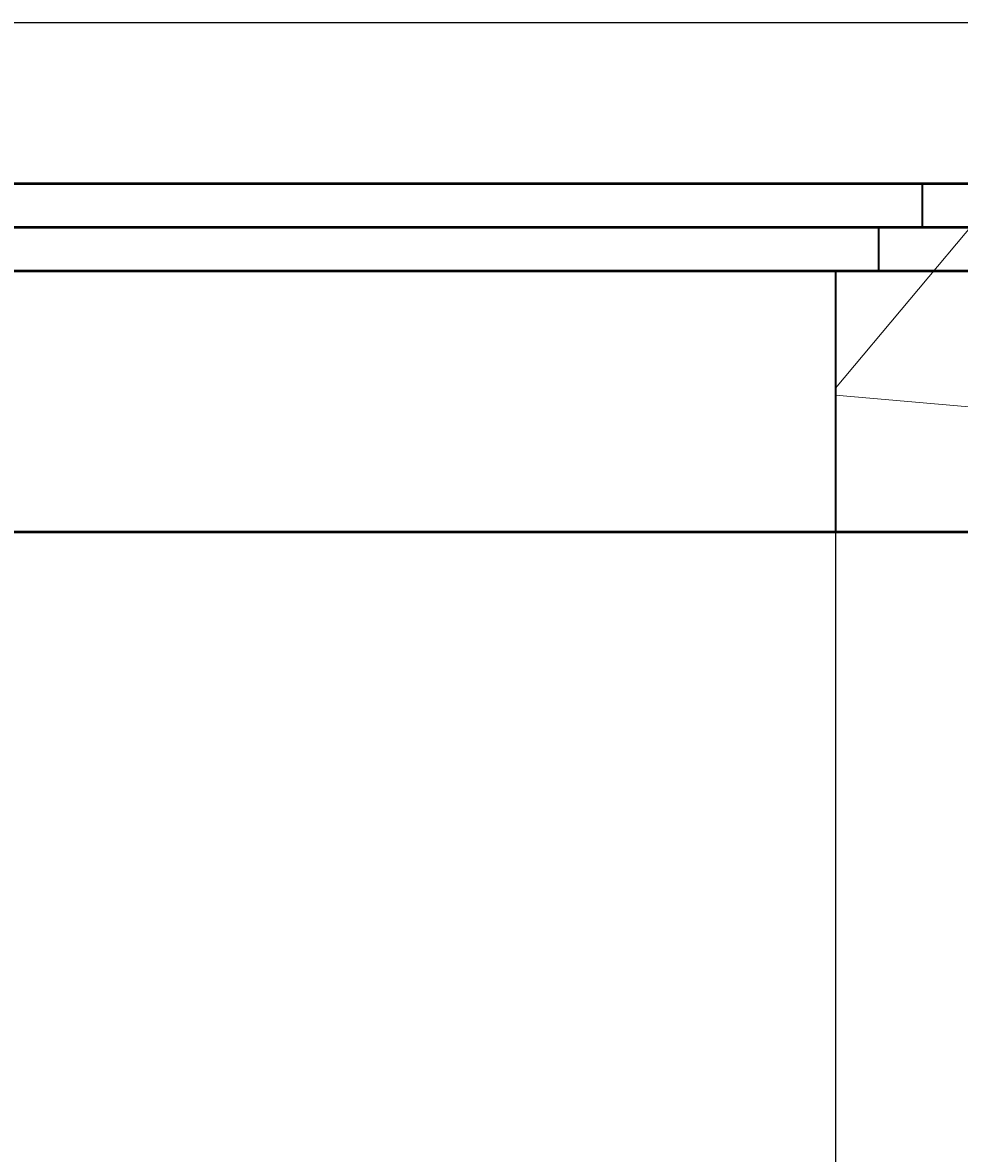
# Model space of a CAD drawing. Units: inches. Extents: x 2812 to 3051, y 1398 to 1659.
# Tile 39 of 65: x 2988 to 3009, y 1468 to 1494. Entities that reach past the tile are written whole.
import ezdxf

# ---------------------------------------------------------------- set-up
doc = ezdxf.new("R2010")
doc.units = ezdxf.units.IN
for name, color, linetype, lineweight in [('A-ANNO-DIMS', 2, 'Continuous', 18), ('S-CONC', 7, 'Continuous', 50), ('S-CONC-PATT', 8, 'Continuous', 18), ('S-CONC-SLAB', 7, 'Continuous', 35)]:
    doc.layers.add(name, color=color, linetype=linetype, lineweight=lineweight)
doc.styles.get("Standard").update_dxf_attribs({"font": 'arial.ttf'})
doc.dimstyles.get("Standard").update_dxf_attribs({"dimtxt": 0.18, "dimasz": 0.18, "dimexe": 0.18, "dimexo": 0.0625, "dimgap": 0.09, "dimtad": 0, "dimtih": 1, "dimtoh": 1, "dimdec": 4, "dimzin": 0, "dimdsep": 46, "dimtxsty": 'Standard', "dimcen": 0.09, "dimadec": 0, "dimazin": 0, "dimtfac": 1, "dimtdec": 4, "dimtofl": 0, "dimtmove": 0, "dimatfit": 3, "dimfxl": 1, "dimtolj": 1, "dimtzin": 0, "dimarcsym": 0})

# ---------------------------------------------------------------- blocks, each defined once
blk = doc.blocks.new('COVER-SLAB-PLAN')
for p, q in [((2, 7), (2, 8)), ((1, 6), (1, 7)), ((1, 7), (2, 7)), ((0, 6), (0, 0)), ((0, 6), (1, 6))]:
    blk.add_line(p, q)
blk = doc.blocks.new('*D47')
at = {"layer": 'A-ANNO-DIMS', "color": 0, "lineweight": -2, "transparency": 16777216}
for p, q in [((2970.385, 1487.973), (2970.385, 1397.505)), ((3006.385, 1487.973), (3006.385, 1397.505)), ((2970.565, 1397.685), (2988.166, 1397.685)), ((3006.205, 1397.685), (2988.604, 1397.685))]:
    blk.add_line(p, q, dxfattribs=at)
at = {"layer": 'A-ANNO-DIMS', "color": 0, "transparency": 16777216}
for points in [[(2970.565, 1397.715), (2970.565, 1397.655), (2970.385, 1397.685)], [(3006.205, 1397.715), (3006.205, 1397.655), (3006.385, 1397.685)]]:
    blk.add_solid(points, dxfattribs=at)
at = {"layer": 'Defpoints', "color": 0, "transparency": 16777216}
for p in [(2970.385, 1488.035), (3006.385, 1488.035), (3006.385, 1397.685)]:
    blk.add_point(p, dxfattribs=at)
at = {"layer": 'A-ANNO-DIMS', "color": 0, "transparency": 16777216, "insert": (2988.385, 1397.685), "char_height": 0.18, "attachment_point": 5}
blk.add_mtext('\\A1;36', dxfattribs=at)
blk = doc.blocks.new('*D48')
at = {"layer": 'A-ANNO-DIMS', "color": 0, "lineweight": -2, "transparency": 16777216}
for p, q in [((3006.385, 1487.973), (3006.385, 1397.505)), ((3036.385, 1409.973), (3036.385, 1397.505)), ((3006.565, 1397.685), (3021.166, 1397.685)), ((3036.205, 1397.685), (3021.603, 1397.685))]:
    blk.add_line(p, q, dxfattribs=at)
at = {"layer": 'A-ANNO-DIMS', "color": 0, "transparency": 16777216}
for points in [[(3006.565, 1397.715), (3006.565, 1397.655), (3006.385, 1397.685)], [(3036.205, 1397.715), (3036.205, 1397.655), (3036.385, 1397.685)]]:
    blk.add_solid(points, dxfattribs=at)
at = {"layer": 'Defpoints', "color": 0, "transparency": 16777216}
for p in [(3006.385, 1488.035), (3036.385, 1410.035), (3036.385, 1397.685)]:
    blk.add_point(p, dxfattribs=at)
at = {"layer": 'A-ANNO-DIMS', "color": 0, "transparency": 16777216, "insert": (3021.385, 1397.685), "char_height": 0.18, "attachment_point": 5}
blk.add_mtext('\\A1;30', dxfattribs=at)
blk = doc.blocks.new('*D55')
at = {"layer": 'A-ANNO-DIMS', "color": 0, "lineweight": -2, "transparency": 16777216}
for p, q in [((2850.811, 1493.738), (3051.178, 1493.738)), ((3050.998, 1493.558), (3050.998, 1491.069)), ((3050.998, 1488.215), (3050.998, 1490.705)), ((2850.811, 1488.035), (3051.178, 1488.035))]:
    blk.add_line(p, q, dxfattribs=at)
at = {"layer": 'A-ANNO-DIMS', "color": 0, "transparency": 16777216}
for points in [[(3050.968, 1493.558), (3051.028, 1493.558), (3050.998, 1493.738)], [(3050.968, 1488.215), (3051.028, 1488.215), (3050.998, 1488.035)]]:
    blk.add_solid(points, dxfattribs=at)
at = {"layer": 'Defpoints', "color": 0, "transparency": 16777216}
for p in [(2850.748, 1493.738), (3050.998, 1493.738), (2850.748, 1488.035)]:
    blk.add_point(p, dxfattribs=at)
at = {"layer": 'A-ANNO-DIMS', "color": 0, "transparency": 16777216, "insert": (3050.998, 1490.887), "char_height": 0.18, "attachment_point": 5}
blk.add_mtext('\\A1;5.703', dxfattribs=at)

msp = doc.modelspace()

# ---------------------------------------------------------------- hatches: boundary and pattern name
at = {"layer": 'S-CONC-PATT'}
h = msp.add_hatch(dxfattribs=at)
h.set_pattern_fill('AR-SAND', color=256, scale=0.3)
h.paths.add_polyline_path([(3036.3849, 1416.0354), (3027.3849, 1416.0354), (2826.3849, 1416.0354), (2826.3849, 1410.0354), (2835.3849, 1410.0354), (3036.3849, 1410.0354)])
h.paths.add_polyline_path([(2970.3849, 1488.0354), (2969.3849, 1488.0354), (2941.3849, 1488.0354), (2941.3849, 1482.0354), (2970.3849, 1482.0354)])
h.paths.add_polyline_path([(3036.3849, 1488.0354), (3035.3849, 1488.0354), (3006.3849, 1488.0354), (3006.3849, 1482.0354), (3027.3849, 1482.0354), (3036.3849, 1482.0354)])
h.paths.add_polyline_path([(3034.3849, 1490.0354), (3008.3849, 1490.0354), (3008.3849, 1489.0354), (3034.3849, 1489.0354)])
h.paths.add_polyline_path([(3035.3849, 1489.0354), (3034.3849, 1489.0354), (3007.3849, 1489.0354), (3007.3849, 1488.0354), (3035.3849, 1488.0354)])
h.paths.add_polyline_path([(2968.3849, 1490.0354), (2943.3849, 1490.0354), (2943.3849, 1489.0354), (2968.3849, 1489.0354)])
h.paths.add_polyline_path([(2969.3849, 1489.0354), (2968.3849, 1489.0354), (2942.3849, 1489.0354), (2942.3849, 1488.0354), (2969.3849, 1488.0354)])
h.paths.add_polyline_path([(2896.3849, 1488.0354), (2826.3849, 1488.0354), (2826.3849, 1482.0354), (2896.3849, 1482.0354)])
h.paths.add_polyline_path([(2895.3849, 1489.0354), (2894.3849, 1489.0354), (2827.3849, 1489.0354), (2827.3849, 1488.0354), (2895.3849, 1488.0354)])
h.paths.add_polyline_path([(2894.3849, 1490.0354), (2828.3849, 1490.0354), (2828.3849, 1489.0354), (2894.3849, 1489.0354)])
h = msp.add_hatch(dxfattribs=at)
h.set_pattern_fill('AR-CONC', color=256, scale=0.3)
h.paths.add_polyline_path([(2896.3849, 1488.0354), (2826.3849, 1488.0354), (2826.3849, 1482.0354), (2896.3849, 1482.0354)])
h.paths.add_polyline_path([(2970.3849, 1488.0354), (2941.3849, 1488.0354), (2941.3849, 1482.0354), (2970.3849, 1482.0354)])
h.paths.add_polyline_path([(2968.3849, 1490.0354), (2943.3849, 1490.0354), (2943.3849, 1489.0354), (2968.3849, 1489.0354)])
h.paths.add_polyline_path([(2969.3849, 1489.0354), (2968.3849, 1489.0354), (2943.3849, 1489.0354), (2942.3849, 1489.0354), (2942.3849, 1488.0354), (2969.3849, 1488.0354)])
h.paths.add_polyline_path([(3036.3849, 1488.0354), (3035.3849, 1488.0354), (3006.3849, 1488.0354), (3006.3849, 1482.0354), (3027.3849, 1482.0354), (3036.3849, 1482.0354)])
h.paths.add_polyline_path([(3035.3849, 1489.0354), (3034.3849, 1489.0354), (3007.3849, 1489.0354), (3007.3849, 1488.0354), (3035.3849, 1488.0354)])
h.paths.add_polyline_path([(3034.3849, 1490.0354), (3008.3849, 1490.0354), (3008.3849, 1489.0354), (3034.3849, 1489.0354)])
h.paths.add_polyline_path([(2895.3849, 1489.0354), (2894.3849, 1489.0354), (2827.3849, 1489.0354), (2827.3849, 1488.0354), (2895.3849, 1488.0354)])
h.paths.add_polyline_path([(2894.3849, 1490.0354), (2828.3849, 1490.0354), (2828.3849, 1489.0354), (2894.3849, 1489.0354)])

# ---------------------------------------------------------------- linework, layer by layer
at = {"layer": 'S-CONC'}
for p, q in [((3034.3849, 1490.0354), (2850.7485, 1490.0354)), ((2850.7485, 1489.0354), (3035.3849, 1489.0354)), ((2850.7485, 1488.0354), (3036.3849, 1488.0354)), ((2850.7485, 1482.0354), (3027.3849, 1482.0354))]:
    msp.add_line(p, q, dxfattribs=at)

# ---------------------------------------------------------------- block references
at = {"layer": 'S-CONC-SLAB'}
msp.add_blockref('COVER-SLAB-PLAN', (3006.385, 1482.035), dxfattribs=at)

# ---------------------------------------------------------------- dimensions: what is measured, and where the dimension line sits
at = {"layer": 'A-ANNO-DIMS'}
dim = msp.add_linear_dim(base=(3050.998, 1493.7383), p1=(2850.7485, 1488.0354), p2=(2850.7485, 1493.7383), angle=90, dimstyle='Standard', override={"dimdec": 3, "dimlfac": 1, "dimrnd": 0, "dimzin": 0, "dimdsep": 46, "dimlunit": 2}, dxfattribs=at)
dim.commit()
dim.dimension.update_dxf_attribs({"geometry": '*D55', "text_midpoint": (3050.998, 1490.8868)})
for base, p1, p2, picture, middle in [((3006.3849, 1397.6854), (2970.3849, 1488.0354), (3006.3849, 1488.0354), '*D47', (2988.3849, 1397.6854)), ((3036.3849, 1397.6854), (3006.3849, 1488.0354), (3036.3849, 1410.0354), '*D48', (3021.3849, 1397.6854))]:
    dim = msp.add_linear_dim(base=base, p1=p1, p2=p2, dimstyle='Standard', override={"dimdec": 0, "dimlfac": 1, "dimrnd": 0, "dimzin": 0, "dimdsep": 46, "dimlunit": 2}, dxfattribs=at)
    dim.commit()
    dim.dimension.update_dxf_attribs({"geometry": picture, "text_midpoint": middle})

doc.saveas('drawing.dxf')
